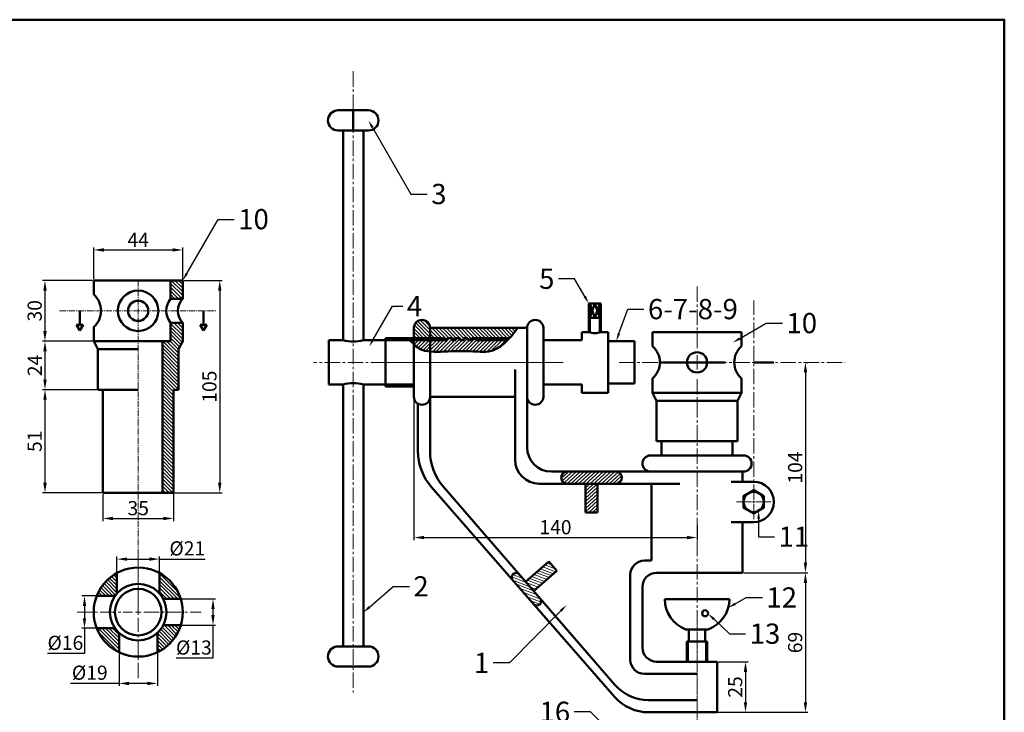
# Model space of a CAD drawing. Units: millimetres. Extents: x 434 to 1535, y -197 to 318.
# Tile 9 of 9: x 1049 to 1535, y -24 to 318. Entities that reach past the tile are written whole.
import ezdxf
from ezdxf import colors
from ezdxf.entities.mleader import LeaderData, LeaderLine
from ezdxf.math import Vec2, Vec3

# ---------------------------------------------------------------- set-up
doc = ezdxf.new("R2010")
doc.units = ezdxf.units.MM
doc.header["$LTSCALE"] = 0.4
doc.linetypes.add('CENTER2', pattern=[28.575, 19.05, -3.175, 3.175, -3.175])
doc.linetypes.add('DASHED', pattern=[19.05, 12.7, -6.35])
for name, color, linetype, lineweight in [('M-CNTR', 1, 'CENTER2', 18), ('M-DIMS', 2, 'Continuous', 25), ('M-HATC', 8, 'Continuous', 18), ('M-HIDN', 6, 'DASHED', 25), ('M-OUTL', 7, 'Continuous', 50), ('M-TEXT', 3, 'Continuous', 25)]:
    doc.layers.add(name, color=color, linetype=linetype, lineweight=lineweight)
doc.styles.get("Standard").update_dxf_attribs({"font": 'arial.ttf'})
doc.dimstyles.new('ISO-25', dxfattribs={"dimtxt": 7, "dimasz": 5, "dimexe": 1.25, "dimexo": 0.625, "dimtad": 1, "dimtoh": 1, "dimdec": 0, "dimtxsty": 'Standard', "dimcen": 2.5, "dimadec": 0, "dimazin": 0, "dimtfac": 1, "dimtdec": 0, "dimtmove": 0, "dimatfit": 3, "dimfxl": 1, "dimarcsym": 0})

# ---------------------------------------------------------------- blocks, each defined once
blk = doc.blocks.new('*U4')
at = {"layer": 'M-CNTR', "color": 0, "transparency": 16777216}
for p, q in [((0, 7), (0, 38.5)), ((-38.5, 0), (-7, 0)), ((7, 0), (73.2, 0)), ((0, -198.75), (0, -7))]:
    blk.add_line(p, q, dxfattribs=at)
at = {"layer": 'M-CNTR', "color": 0, "linetype": 'Continuous', "transparency": 16777216}
for p, q in [((-3.5, 0), (3.5, 0)), ((0, -3.5), (0, 3.5))]:
    blk.add_line(p, q, dxfattribs=at)
blk = doc.blocks.new('*U5')
at = {"layer": 'M-CNTR', "color": 0, "transparency": 16777216}
for p, q in [((0, 1), (0, 99.51)), ((-8.5, 0), (-1, 0)), ((1, 0), (8.5, 0)), ((0, -8.5), (0, -1))]:
    blk.add_line(p, q, dxfattribs=at)
at = {"layer": 'M-CNTR', "color": 0, "linetype": 'Continuous', "transparency": 16777216}
for p, q in [((-0.5, 0), (0.5, 0)), ((0, -0.5), (0, 0.5))]:
    blk.add_line(p, q, dxfattribs=at)
blk = doc.blocks.new('*U6')
at = {"layer": 'M-CNTR', "color": 0, "transparency": 16777216}
blk.add_line((-44.39, 0), (44.11, 0), dxfattribs=at)
blk = doc.blocks.new('*U46')
at = {"layer": 'M-CNTR', "color": 0, "transparency": 16777216}
blk.add_line((33.1, 0), (-82.84, 0), dxfattribs=at)
blk = doc.blocks.new('*U47')
at = {"layer": 'M-CNTR', "color": 0, "transparency": 16777216}
blk.add_line((0, 81.09), (0, -225.98), dxfattribs=at)
blk = doc.blocks.new('*U80')
at = {"layer": 'M-CNTR', "color": 0, "transparency": 16777216}
blk.add_line((0, -17.2), (0, 69.52), dxfattribs=at)
blk = doc.blocks.new('*D102')
at = {"layer": 'Defpoints', "color": 0, "ltscale": 0.4, "transparency": 16777216}
for p in [(1129.22, 204.63), (1085.22, 189.54), (1129.22, 189.54)]:
    blk.add_point(p, dxfattribs=at)
at = {"layer": 'M-DIMS', "color": 0, "lineweight": -2, "ltscale": 0.4, "transparency": 16777216}
for p, q in [((1085.22, 190.17), (1085.22, 205.88)), ((1090.22, 204.63), (1124.22, 204.63)), ((1129.22, 190.17), (1129.22, 205.88))]:
    blk.add_line(p, q, dxfattribs=at)
at = {"layer": 'M-DIMS', "color": 0, "ltscale": 0.4, "transparency": 16777216}
for points in [[(1090.22, 205.46), (1090.22, 203.79), (1085.22, 204.63)], [(1124.22, 205.46), (1124.22, 203.79), (1129.22, 204.63)]]:
    blk.add_solid(points, dxfattribs=at)
at = {"layer": 'M-DIMS', "color": 0, "ltscale": 0.4, "transparency": 16777216, "insert": (1107.22, 208.75), "char_height": 7, "attachment_point": 5}
blk.add_mtext('44', dxfattribs=at)
blk = doc.blocks.new('*D103')
at = {"layer": 'Defpoints', "color": 0, "ltscale": 0.4, "transparency": 16777216}
for p in [(1089.72, 84.54), (1124.72, 84.54), (1124.72, 71.88)]:
    blk.add_point(p, dxfattribs=at)
at = {"layer": 'M-DIMS', "color": 0, "lineweight": -2, "ltscale": 0.4, "transparency": 16777216}
for p, q in [((1089.72, 83.92), (1089.72, 70.63)), ((1124.72, 83.92), (1124.72, 70.63)), ((1094.72, 71.88), (1119.72, 71.88))]:
    blk.add_line(p, q, dxfattribs=at)
at = {"layer": 'M-DIMS', "color": 0, "ltscale": 0.4, "transparency": 16777216}
for points in [[(1094.72, 72.71), (1094.72, 71.05), (1089.72, 71.88)], [(1119.72, 72.71), (1119.72, 71.05), (1124.72, 71.88)]]:
    blk.add_solid(points, dxfattribs=at)
at = {"layer": 'M-DIMS', "color": 0, "ltscale": 0.4, "transparency": 16777216, "insert": (1107.22, 76.08), "char_height": 7, "attachment_point": 5}
blk.add_mtext('35', dxfattribs=at)
blk = doc.blocks.new('*D104')
at = {"layer": 'Defpoints', "color": 0, "ltscale": 0.4, "transparency": 16777216}
for p in [(1085.22, 189.54), (1061.12, 159.54), (1085.22, 159.54)]:
    blk.add_point(p, dxfattribs=at)
at = {"layer": 'M-DIMS', "color": 0, "lineweight": -2, "ltscale": 0.4, "transparency": 16777216}
for p, q in [((1084.6, 189.54), (1059.87, 189.54)), ((1061.12, 184.54), (1061.12, 164.54)), ((1084.6, 159.54), (1059.87, 159.54))]:
    blk.add_line(p, q, dxfattribs=at)
at = {"layer": 'M-DIMS', "color": 0, "ltscale": 0.4, "transparency": 16777216}
for points in [[(1060.29, 184.54), (1061.96, 184.54), (1061.12, 189.54)], [(1060.29, 164.54), (1061.96, 164.54), (1061.12, 159.54)]]:
    blk.add_solid(points, dxfattribs=at)
at = {"layer": 'M-DIMS', "color": 0, "ltscale": 0.4, "transparency": 16777216, "insert": (1056.92, 174.54), "char_height": 7, "attachment_point": 5, "rotation": 90}
blk.add_mtext('30', dxfattribs=at)
blk = doc.blocks.new('*D105')
at = {"layer": 'Defpoints', "color": 0, "ltscale": 0.4, "transparency": 16777216}
for p in [(1085.22, 159.54), (1061.12, 135.54), (1087.22, 135.54)]:
    blk.add_point(p, dxfattribs=at)
at = {"layer": 'M-DIMS', "color": 0, "lineweight": -2, "ltscale": 0.4, "transparency": 16777216}
for p, q in [((1084.6, 159.54), (1059.87, 159.54)), ((1061.12, 154.54), (1061.12, 140.54)), ((1086.6, 135.54), (1059.87, 135.54))]:
    blk.add_line(p, q, dxfattribs=at)
at = {"layer": 'M-DIMS', "color": 0, "ltscale": 0.4, "transparency": 16777216}
for points in [[(1060.29, 154.54), (1061.96, 154.54), (1061.12, 159.54)], [(1060.29, 140.54), (1061.96, 140.54), (1061.12, 135.54)]]:
    blk.add_solid(points, dxfattribs=at)
at = {"layer": 'M-DIMS', "color": 0, "ltscale": 0.4, "transparency": 16777216, "insert": (1056.98, 147.54), "char_height": 7, "attachment_point": 5, "rotation": 90}
blk.add_mtext('24', dxfattribs=at)
blk = doc.blocks.new('*D101')
at = {"layer": 'Defpoints', "color": 0, "ltscale": 0.4, "transparency": 16777216}
for p in [(1087.22, 135.54), (1061.12, 84.54), (1089.72, 84.54)]:
    blk.add_point(p, dxfattribs=at)
at = {"layer": 'M-DIMS', "color": 0, "lineweight": -2, "ltscale": 0.4, "transparency": 16777216}
for p, q in [((1086.6, 135.54), (1059.87, 135.54)), ((1061.12, 130.54), (1061.12, 89.54)), ((1089.1, 84.54), (1059.87, 84.54))]:
    blk.add_line(p, q, dxfattribs=at)
at = {"layer": 'M-DIMS', "color": 0, "ltscale": 0.4, "transparency": 16777216}
for points in [[(1060.29, 130.54), (1061.96, 130.54), (1061.12, 135.54)], [(1060.29, 89.54), (1061.96, 89.54), (1061.12, 84.54)]]:
    blk.add_solid(points, dxfattribs=at)
at = {"layer": 'M-DIMS', "color": 0, "ltscale": 0.4, "transparency": 16777216, "insert": (1056.92, 110.04), "char_height": 7, "attachment_point": 5, "rotation": 90}
blk.add_mtext('51', dxfattribs=at)
blk = doc.blocks.new('*D106')
at = {"layer": 'Defpoints', "color": 0, "ltscale": 0.4, "transparency": 16777216}
for p in [(1129.22, 189.54), (1119.22, 84.54), (1147.54, 84.54)]:
    blk.add_point(p, dxfattribs=at)
at = {"layer": 'M-DIMS', "color": 0, "lineweight": -2, "ltscale": 0.4, "transparency": 16777216}
for p, q in [((1129.85, 189.54), (1148.79, 189.54)), ((1147.54, 184.54), (1147.54, 89.54)), ((1119.85, 84.54), (1148.79, 84.54))]:
    blk.add_line(p, q, dxfattribs=at)
at = {"layer": 'M-DIMS', "color": 0, "ltscale": 0.4, "transparency": 16777216}
for points in [[(1146.71, 184.54), (1148.38, 184.54), (1147.54, 189.54)], [(1146.71, 89.54), (1148.38, 89.54), (1147.54, 84.54)]]:
    blk.add_solid(points, dxfattribs=at)
at = {"layer": 'M-DIMS', "color": 0, "ltscale": 0.4, "transparency": 16777216, "insert": (1143.34, 137.04), "char_height": 7, "attachment_point": 5, "rotation": 90}
blk.add_mtext('105', dxfattribs=at)
blk = doc.blocks.new('*U100')
at = {"layer": 'M-CNTR', "color": 0, "transparency": 16777216}
for p, q in [((0, 2.8), (0, 28.76)), ((-30.25, 0), (-2.8, 0)), ((2.8, 0), (31.18, 0)), ((0, -32.64), (0, -2.8))]:
    blk.add_line(p, q, dxfattribs=at)
at = {"layer": 'M-CNTR', "color": 0, "linetype": 'Continuous', "transparency": 16777216}
for p, q in [((-1.4, 0), (1.4, 0)), ((0, -1.4), (0, 1.4))]:
    blk.add_line(p, q, dxfattribs=at)
blk = doc.blocks.new('*D107')
at = {"layer": 'Defpoints', "color": 0, "ltscale": 0.4, "transparency": 16777216}
for p in [(1117.72, 51.8), (1096.72, 44.92), (1117.72, 44.92)]:
    blk.add_point(p, dxfattribs=at)
at = {"layer": 'M-DIMS', "color": 0, "lineweight": -2, "ltscale": 0.4, "transparency": 16777216}
for p, q in [((1096.72, 45.55), (1096.72, 53.05)), ((1101.72, 51.8), (1112.72, 51.8)), ((1117.72, 45.55), (1117.72, 53.05)), ((1117.72, 51.8), (1140.26, 51.8))]:
    blk.add_line(p, q, dxfattribs=at)
at = {"layer": 'M-DIMS', "color": 0, "ltscale": 0.4, "transparency": 16777216}
for points in [[(1101.72, 52.63), (1101.72, 50.96), (1096.72, 51.8)], [(1112.72, 52.63), (1112.72, 50.96), (1117.72, 51.8)]]:
    blk.add_solid(points, dxfattribs=at)
at = {"layer": 'M-DIMS', "color": 0, "ltscale": 0.4, "transparency": 16777216, "insert": (1131.49, 56.19), "char_height": 7, "attachment_point": 5}
blk.add_mtext('%%C21', dxfattribs=at)
blk = doc.blocks.new('*D108')
at = {"layer": 'Defpoints', "color": 0, "ltscale": 0.4, "transparency": 16777216}
for p in [(1128.24, 32.09), (1128.24, 19.09), (1144.19, 19.09)]:
    blk.add_point(p, dxfattribs=at)
at = {"layer": 'M-DIMS', "color": 0, "lineweight": -2, "ltscale": 0.4, "transparency": 16777216}
for p, q in [((1128.86, 32.09), (1145.44, 32.09)), ((1144.19, 27.09), (1144.19, 24.09)), ((1128.86, 19.09), (1145.44, 19.09)), ((1144.19, 19.09), (1144.19, 2.78)), ((1144.19, 2.78), (1125.92, 2.78))]:
    blk.add_line(p, q, dxfattribs=at)
at = {"layer": 'M-DIMS', "color": 0, "ltscale": 0.4, "transparency": 16777216}
for points in [[(1143.36, 27.09), (1145.02, 27.09), (1144.19, 32.09)], [(1143.36, 24.09), (1145.02, 24.09), (1144.19, 19.09)]]:
    blk.add_solid(points, dxfattribs=at)
at = {"layer": 'M-DIMS', "color": 0, "ltscale": 0.4, "transparency": 16777216, "insert": (1134.74, 7.18), "char_height": 7, "attachment_point": 5}
blk.add_mtext('%%C13', dxfattribs=at)
blk = doc.blocks.new('*D109')
at = {"layer": 'Defpoints', "color": 0, "ltscale": 0.4, "transparency": 16777216}
for p in [(1086.73, 33.59), (1080.65, 17.59), (1086.73, 17.59)]:
    blk.add_point(p, dxfattribs=at)
at = {"layer": 'M-DIMS', "color": 0, "lineweight": -2, "ltscale": 0.4, "transparency": 16777216}
for p, q in [((1086.1, 33.59), (1079.4, 33.59)), ((1080.65, 28.59), (1080.65, 22.59)), ((1086.1, 17.59), (1079.4, 17.59)), ((1080.65, 17.59), (1080.65, 5.11)), ((1080.65, 5.11), (1062.39, 5.11))]:
    blk.add_line(p, q, dxfattribs=at)
at = {"layer": 'M-DIMS', "color": 0, "ltscale": 0.4, "transparency": 16777216}
for points in [[(1079.82, 28.59), (1081.48, 28.59), (1080.65, 33.59)], [(1079.82, 22.59), (1081.48, 22.59), (1080.65, 17.59)]]:
    blk.add_solid(points, dxfattribs=at)
at = {"layer": 'M-DIMS', "color": 0, "ltscale": 0.4, "transparency": 16777216, "insert": (1071.21, 9.5), "char_height": 7, "attachment_point": 5}
blk.add_mtext('%%C16', dxfattribs=at)
blk = doc.blocks.new('*D110')
at = {"layer": 'Defpoints', "color": 0, "ltscale": 0.4, "transparency": 16777216}
for p in [(1097.72, 5.75), (1116.72, 5.75), (1116.72, -9.67)]:
    blk.add_point(p, dxfattribs=at)
at = {"layer": 'M-DIMS', "color": 0, "lineweight": -2, "ltscale": 0.4, "transparency": 16777216}
for p, q in [((1097.72, 5.12), (1097.72, -10.92)), ((1116.72, 5.12), (1116.72, -10.92)), ((1097.72, -9.67), (1073.81, -9.67)), ((1111.72, -9.67), (1102.72, -9.67))]:
    blk.add_line(p, q, dxfattribs=at)
at = {"layer": 'M-DIMS', "color": 0, "ltscale": 0.4, "transparency": 16777216}
for points in [[(1102.72, -8.83), (1102.72, -10.5), (1097.72, -9.67)], [(1111.72, -8.83), (1111.72, -10.5), (1116.72, -9.67)]]:
    blk.add_solid(points, dxfattribs=at)
at = {"layer": 'M-DIMS', "color": 0, "ltscale": 0.4, "transparency": 16777216, "insert": (1083.27, -5.27), "char_height": 7, "attachment_point": 5}
blk.add_mtext('%%C19', dxfattribs=at)
blk = doc.blocks.new('*D127')
at = {"layer": 'Defpoints', "color": 0, "ltscale": 0.4, "transparency": 16777216}
for p in [(1436.75, 149.06), (1406.04, 45.06), (1437.14, 45.06)]:
    blk.add_point(p, dxfattribs=at)
at = {"layer": 'M-DIMS', "color": 0, "lineweight": -2, "ltscale": 0.4, "transparency": 16777216}
for p, q in [((1437.38, 149.06), (1438.39, 149.06)), ((1437.14, 144.06), (1437.14, 50.06)), ((1406.66, 45.06), (1438.39, 45.06))]:
    blk.add_line(p, q, dxfattribs=at)
at = {"layer": 'M-DIMS', "color": 0, "ltscale": 0.4, "transparency": 16777216}
for points in [[(1436.31, 144.06), (1437.98, 144.06), (1437.14, 149.06)], [(1436.31, 50.06), (1437.98, 50.06), (1437.14, 45.06)]]:
    blk.add_solid(points, dxfattribs=at)
at = {"layer": 'M-DIMS', "color": 0, "ltscale": 0.4, "transparency": 16777216, "insert": (1432.95, 97.06), "char_height": 7, "attachment_point": 5, "rotation": 90}
blk.add_mtext('104', dxfattribs=at)
blk = doc.blocks.new('*D128')
at = {"layer": 'Defpoints', "color": 0, "ltscale": 0.4, "transparency": 16777216}
for p in [(1406.04, 45.06), (1383.54, -23.94), (1437.14, -23.94)]:
    blk.add_point(p, dxfattribs=at)
at = {"layer": 'M-DIMS', "color": 0, "lineweight": -2, "ltscale": 0.4, "transparency": 16777216}
for p, q in [((1406.66, 45.06), (1438.39, 45.06)), ((1437.14, 40.06), (1437.14, -18.94)), ((1384.16, -23.94), (1438.39, -23.94))]:
    blk.add_line(p, q, dxfattribs=at)
at = {"layer": 'M-DIMS', "color": 0, "ltscale": 0.4, "transparency": 16777216}
for points in [[(1436.31, 40.06), (1437.98, 40.06), (1437.14, 45.06)], [(1436.31, -18.94), (1437.98, -18.94), (1437.14, -23.94)]]:
    blk.add_solid(points, dxfattribs=at)
at = {"layer": 'M-DIMS', "color": 0, "ltscale": 0.4, "transparency": 16777216, "insert": (1432.95, 10.56), "char_height": 7, "attachment_point": 5, "rotation": 90}
blk.add_mtext('69', dxfattribs=at)
blk = doc.blocks.new('*D129')
at = {"layer": 'Defpoints', "color": 0, "ltscale": 0.4, "transparency": 16777216}
for p in [(1393.54, 1.06), (1393.54, -23.94), (1407.51, -23.94)]:
    blk.add_point(p, dxfattribs=at)
at = {"layer": 'M-DIMS', "color": 0, "lineweight": -2, "ltscale": 0.4, "transparency": 16777216}
for p, q in [((1394.16, 1.06), (1408.76, 1.06)), ((1407.51, -3.94), (1407.51, -18.94)), ((1394.16, -23.94), (1408.76, -23.94))]:
    blk.add_line(p, q, dxfattribs=at)
at = {"layer": 'M-DIMS', "color": 0, "ltscale": 0.4, "transparency": 16777216}
for points in [[(1406.67, -3.94), (1408.34, -3.94), (1407.51, 1.06)], [(1406.67, -18.94), (1408.34, -18.94), (1407.51, -23.94)]]:
    blk.add_solid(points, dxfattribs=at)
at = {"layer": 'M-DIMS', "color": 0, "ltscale": 0.4, "transparency": 16777216, "insert": (1403.31, -11.44), "char_height": 7, "attachment_point": 5, "rotation": 90}
blk.add_mtext('25', dxfattribs=at)
blk = doc.blocks.new('*D130')
at = {"layer": 'Defpoints', "color": 0, "ltscale": 0.4, "transparency": 16777216}
for p in [(1243.54, 137.06), (1383.54, 69.2), (1383.54, 62.45)]:
    blk.add_point(p, dxfattribs=at)
at = {"layer": 'M-DIMS', "color": 0, "lineweight": -2, "ltscale": 0.4, "transparency": 16777216}
for p, q in [((1243.54, 136.43), (1243.54, 61.2)), ((1383.54, 68.57), (1383.54, 61.2)), ((1248.54, 62.45), (1378.54, 62.45))]:
    blk.add_line(p, q, dxfattribs=at)
at = {"layer": 'M-DIMS', "color": 0, "ltscale": 0.4, "transparency": 16777216}
for points in [[(1248.54, 63.28), (1248.54, 61.62), (1243.54, 62.45)], [(1378.54, 63.28), (1378.54, 61.62), (1383.54, 62.45)]]:
    blk.add_solid(points, dxfattribs=at)
at = {"layer": 'M-DIMS', "color": 0, "ltscale": 0.4, "transparency": 16777216, "insert": (1313.54, 66.65), "char_height": 7, "attachment_point": 5}
blk.add_mtext('140', dxfattribs=at)
blk = doc.blocks.new('DIE')
at = {"ltscale": 0.4}
for p, q in [((0, 15), (32, 15)), ((21.57, 0), (10.43, 0))]:
    blk.add_line(p, q, dxfattribs=at)
for start, end in [(180, 249.6359), (290.3641, 0)]:
    blk.add_arc((16, 15), 16, start, end, dxfattribs=at)

msp = doc.modelspace()

# ---------------------------------------------------------------- hatches: boundary and pattern name
at = {"layer": 'M-HATC', "ltscale": 0.4}
h = msp.add_hatch(dxfattribs=at)
h.set_pattern_fill('ANSI31', color=256, scale=0.4, angle=90)
h.set_pattern_definition([(135, (-60.0056, 264.9336), (-0.8980256, -0.8980256), [])])
h.paths.add_polyline_path([(1119.22, 84.54), (1124.72, 84.54), (1124.72, 135.54), (1127.22, 135.54), (1127.22, 155.54), (1129.22, 159.54), (1129.22, 168.54), (1123.22, 168.54), (1123.22, 159.54), (1119.22, 159.54)])
h.paths.add_polyline_path([(1129.22, 189.54), (1123.22, 189.54), (1123.22, 180.54), (1129.22, 180.54)])
h = msp.add_hatch(dxfattribs=at)
h.set_pattern_fill('ANSI31', color=256, scale=0.4, angle=90)
h.set_pattern_definition([(135, (1944.4597, -517.0887), (-0.8980256, -0.8980256), [])])
edge = h.paths.add_edge_path()
edge.add_line((1251.54, 166.06), (1251.54, 161.06))
edge.add_line((1251.54, 161.06), (1258.22, 161.06))
edge.add_line((1258.22, 161.06), (1290.81, 161.06))
edge.add_spline(control_points=[(1290.81, 161.06), (1292.23, 162.63), (1293.6, 164.34), (1294.97, 166.06)], knot_values=[54.490486, 54.490486, 54.490486, 54.490486, 60.411943, 60.411943, 60.411943, 60.411943], degree=3, periodic=0)
edge.add_line((1294.97, 166.06), (1251.54, 166.06))
h.paths.add_polyline_path([(1251.54, 166.06, 1), (1243.54, 166.06), (1243.54, 161.06), (1251.54, 161.06)])
h = msp.add_hatch(dxfattribs=at)
h.set_pattern_fill('ANSI31', color=256, scale=0.4)
h.set_pattern_definition([(45, (1944.4597, -517.0887), (-0.8980256, 0.8980256), [])])
edge = h.paths.add_edge_path()
edge.add_spline(control_points=[(1251.54, 154.39), (1253.75, 154.19), (1261.99, 154.61), (1271.04, 154.74), (1282.58, 153.83), (1287.09, 157.16), (1289.88, 160.06)], knot_values=[13.163081, 13.163081, 13.163081, 13.163081, 19.718754, 36.150911, 41.776837, 53.205274, 53.205274, 53.205274, 53.205274], degree=3, periodic=0)
edge.add_line((1289.88, 160.06), (1278.04, 160.06))
edge.add_spline(control_points=[(1278.04, 160.06), (1277.22, 159.19), (1275.16, 156.98), (1270.08, 158.14), (1265.21, 158.03), (1260.18, 157.28), (1257.67, 159.16), (1256.48, 160.06)], knot_values=[0, 0, 0, 0, 3.382531, 8.59366, 13.864007, 18.596096, 22.91005, 22.91005, 22.91005, 22.91005], degree=3, periodic=0)
edge.add_line((1256.48, 160.06), (1251.54, 160.06))
edge.add_line((1251.54, 160.06), (1251.54, 154.39))
edge = h.paths.add_edge_path()
edge.add_line((1251.54, 160.06), (1243.54, 160.06))
edge.add_line((1243.54, 160.06), (1243.54, 157.99))
edge.add_spline(control_points=[(1243.54, 157.99), (1244.35, 157.17), (1246.66, 155.25), (1249.6, 154.57), (1251.54, 154.39)], knot_values=[3.982747, 3.982747, 3.982747, 3.982747, 7.427781, 13.163081, 13.163081, 13.163081, 13.163081], degree=3, periodic=0)
edge.add_line((1251.54, 154.39), (1251.54, 160.06))
edge = h.paths.add_edge_path()
edge.add_spline(control_points=[(1256.48, 160.06), (1257.67, 159.16), (1260.18, 157.28), (1265.21, 158.03), (1270.08, 158.14), (1275.16, 156.98), (1277.22, 159.19), (1278.04, 160.06)], knot_values=[0, 0, 0, 0, 4.313954, 9.046043, 14.31639, 19.527519, 22.91005, 22.91005, 22.91005, 22.91005], degree=3, periodic=0)
edge.add_line((1278.04, 160.06), (1274.22, 160.06))
edge.add_line((1274.22, 160.06), (1274.22, 161.06))
edge.add_line((1274.22, 161.06), (1272.22, 161.06))
edge.add_line((1272.22, 161.06), (1272.22, 160.06))
edge.add_line((1272.22, 160.06), (1270.22, 160.06))
edge.add_line((1270.22, 160.06), (1270.22, 161.06))
edge.add_line((1270.22, 161.06), (1268.22, 161.06))
edge.add_line((1268.22, 161.06), (1268.22, 160.06))
edge.add_line((1268.22, 160.06), (1266.22, 160.06))
edge.add_line((1266.22, 160.06), (1266.22, 161.06))
edge.add_line((1266.22, 161.06), (1264.22, 161.06))
edge.add_line((1264.22, 161.06), (1264.22, 160.06))
edge.add_line((1264.22, 160.06), (1262.22, 160.06))
edge.add_line((1262.22, 160.06), (1262.22, 161.06))
edge.add_line((1262.22, 161.06), (1260.22, 161.06))
edge.add_line((1260.22, 161.06), (1260.22, 160.06))
edge.add_line((1260.22, 160.06), (1258.22, 160.06))
edge.add_line((1258.22, 160.06), (1256.48, 160.06))
h = msp.add_hatch(dxfattribs=at)
h.set_pattern_fill('ANSI31', color=256, scale=0.4, angle=177)
h.set_pattern_definition([(222, (735.9605, -22.5014), (0.8497959, -0.943794), [])])
h.paths.add_polyline_path([(1343.38, 95.06), (1319.38, 95.06, 1), (1319.38, 89.06), (1343.38, 89.06, 1)])
h.paths.add_polyline_path([(1334.38, 89.06), (1328.38, 89.06), (1328.38, 74.88), (1334.38, 74.88)])
h = msp.add_hatch(dxfattribs=at)
h.set_pattern_fill('ANSI31', color=256, scale=0.4, angle=114)
h.set_pattern_definition([(159, (735.9605, -22.5014), (-0.4551273, -1.1856471), [])])
h.paths.add_polyline_path([(1314.18, 46.03), (1310.23, 50.54), (1298.8, 40.56), (1302.74, 36.02)])
h.paths.add_polyline_path([(1302.78, 29.56, 0.998098), (1305.95, 32.32), (1295.62, 44.23, 1.001905), (1292.4, 41.43)])
h = msp.add_hatch(dxfattribs=at)
h.set_pattern_fill('ANSI31', color=256, scale=0.4, angle=90)
h.set_pattern_definition([(135, (-250.1834, 254.1624), (-0.8980256, -0.8980256), [])])
h.paths.add_polyline_path([(1128.24, 32.09, 0.195774), (1117.72, 44.92), (1117.72, 34.85, -0.060049), (1119.62, 32.09)])
h.paths.add_polyline_path([(1086.73, 33.59), (1095.73, 33.59, -0.02863), (1096.72, 34.85), (1096.72, 44.92, 0.177087)])
h.paths.add_polyline_path([(1097.72, 5.75), (1097.72, 15.31, -0.054237), (1095.73, 17.59), (1086.73, 17.59, 0.190278)])
h.paths.add_polyline_path([(1116.72, 5.75, 0.209058), (1128.24, 19.09), (1119.62, 19.09, -0.085747), (1116.72, 15.31)])

# ---------------------------------------------------------------- linework, layer by layer
at = {"layer": 'M-CNTR', "ltscale": 0.4}
for p, q in [((1107.22, 189.54), (1107.22, 25.59)), ((1068.34, 174.54), (1145.99, 174.54))]:
    msp.add_line(p, q, dxfattribs=at)
at = {"layer": 'M-HIDN', "ltscale": 0.4}
msp.add_line((1243.54, 161.06), (1290.81, 161.06), dxfattribs=at)
at = {"layer": 'M-OUTL', "ltscale": 0.4}
for p, q in [((1213.54, 273.67), (1213.54, 263.67)), ((1213.54, 263.67), (1208.54, 263.67)), ((1208.54, 263.67), (1208.54, 160.06)), ((1213.54, 263.67), (1218.54, 263.67)), ((1218.54, 263.67), (1218.54, 160.06)), ((1085.22, 189.54), (1129.22, 189.54)), ((1085.22, 182.54), (1085.22, 189.54)), ((1123.22, 180.54), (1123.22, 189.54)), ((1129.22, 189.54), (1129.22, 180.54)), ((1129.22, 180.54), (1123.22, 180.54)), ((1330.04, 178.14), (1330.04, 164.06)), ((1336.04, 178.14), (1330.04, 178.14)), ((1330.54, 178.14), (1330.54, 163.88)), ((1333.04, 171.14), (1330.54, 178.14)), ((1333.04, 178.14), (1330.54, 171.14)), ((1335.54, 178.14), (1333.04, 171.14)), ((1333.04, 178.14), (1335.54, 171.14)), ((1335.54, 163.88), (1335.54, 178.14)), ((1336.04, 164.06), (1336.04, 178.14)), ((1078.4, 174.54), (1078.4, 167.67)), ((1139.57, 174.54), (1139.57, 167.67)), ((1336.04, 171.14), (1330.04, 171.14)), ((1078.4, 164.8), (1076.74, 167.67)), ((1076.74, 167.67), (1080.05, 167.67)), ((1078.4, 164.8), (1080.05, 167.67)), ((1085.22, 159.54), (1085.22, 166.54)), ((1123.22, 159.54), (1123.22, 168.54)), ((1129.22, 168.54), (1123.22, 168.54)), ((1129.22, 168.54), (1129.22, 159.54)), ((1139.57, 164.8), (1137.91, 167.67)), ((1137.91, 167.67), (1141.23, 167.67)), ((1139.57, 164.8), (1141.23, 167.67)), ((1243.54, 132.06), (1243.54, 166.06)), ((1251.54, 166.06), (1251.54, 132.06)), ((1251.54, 166.06), (1299.54, 166.06)), ((1299.54, 132.06), (1299.54, 166.06)), ((1307.54, 166.06), (1307.54, 132.06)), ((1229.54, 161.06), (1229.54, 137.06)), ((1258.22, 161.06), (1229.54, 161.06)), ((1258.22, 161.06), (1258.22, 160.06)), ((1262.22, 161.06), (1260.22, 161.06)), ((1260.22, 160.06), (1260.22, 161.06)), ((1262.22, 161.06), (1262.22, 160.06)), ((1266.22, 161.06), (1264.22, 161.06)), ((1264.22, 160.06), (1264.22, 161.06)), ((1264.22, 161.06), (1266.22, 161.06)), ((1266.22, 161.06), (1266.22, 160.06)), ((1270.22, 161.06), (1268.22, 161.06)), ((1268.22, 160.06), (1268.22, 161.06)), ((1268.22, 161.06), (1270.22, 161.06)), ((1270.22, 161.06), (1270.22, 160.06)), ((1290.81, 161.06), (1272.22, 161.06)), ((1272.22, 160.06), (1272.22, 161.06)), ((1272.22, 161.06), (1274.22, 161.06)), ((1274.22, 161.06), (1274.22, 160.06)), ((1299.54, 137.06), (1299.54, 161.06)), ((1326.54, 164.06), (1326.54, 160.06)), ((1330.04, 164.06), (1326.54, 164.06)), ((1339.54, 164.06), (1336.04, 164.06)), ((1339.54, 149.06), (1339.54, 164.06)), ((1361.54, 164.06), (1405.54, 164.06)), ((1361.54, 157.06), (1361.54, 164.06)), ((1405.54, 164.06), (1405.54, 157.06)), ((1123.22, 159.54), (1085.22, 159.54)), ((1085.22, 159.54), (1087.22, 155.54)), ((1119.22, 159.54), (1119.22, 84.54)), ((1129.22, 159.54), (1127.22, 155.54)), ((1208.54, 160.06), (1201.54, 160.06)), ((1201.54, 160.06), (1201.54, 138.06)), ((1229.54, 160.06), (1218.54, 160.06)), ((1260.22, 160.06), (1229.54, 160.06)), ((1258.22, 160.06), (1260.22, 160.06)), ((1264.22, 160.06), (1262.22, 160.06)), ((1262.22, 160.06), (1264.22, 160.06)), ((1268.22, 160.06), (1266.22, 160.06)), ((1266.22, 160.06), (1268.22, 160.06)), ((1272.22, 160.06), (1270.22, 160.06)), ((1270.22, 160.06), (1272.22, 160.06)), ((1289.88, 160.06), (1274.22, 160.06)), ((1326.54, 160.06), (1307.54, 160.06)), ((1339.54, 159.56), (1339.54, 138.56)), ((1339.54, 159.56), (1352.54, 159.56)), ((1352.54, 138.56), (1352.54, 159.56)), ((1107.22, 155.54), (1087.22, 155.54)), ((1087.22, 135.54), (1087.22, 155.54)), ((1127.22, 155.54), (1127.22, 135.54)), ((1339.54, 134.06), (1339.54, 149.06)), ((1365.15, 149.06), (1397.42, 149.06)), ((1293.54, 145.49), (1293.54, 101.06)), ((1201.54, 138.06), (1208.54, 138.06)), ((1208.54, 138.06), (1208.54, 8.67)), ((1218.54, 138.06), (1229.54, 138.06)), ((1218.54, 138.06), (1218.54, 8.67)), ((1229.54, 138.06), (1243.54, 138.06)), ((1229.54, 137.06), (1243.54, 137.06)), ((1307.54, 138.06), (1326.54, 138.06)), ((1326.54, 138.06), (1326.54, 134.06)), ((1339.54, 138.56), (1352.54, 138.56)), ((1361.54, 134.06), (1361.54, 141.06)), ((1405.54, 134.06), (1405.54, 141.06)), ((1107.22, 135.54), (1087.22, 135.54)), ((1089.72, 135.54), (1089.72, 84.54)), ((1127.22, 135.54), (1124.72, 135.54)), ((1124.72, 135.54), (1124.72, 84.54)), ((1251.54, 132.06), (1293.54, 132.06)), ((1251.54, 105.14), (1251.54, 132.06)), ((1299.54, 132.06), (1299.54, 107.06)), ((1326.54, 134.06), (1339.54, 134.06)), ((1339.54, 134.06), (1333.54, 134.06)), ((1405.54, 134.06), (1361.54, 134.06)), ((1361.54, 134.06), (1363.54, 130.06)), ((1405.54, 134.06), (1403.54, 130.06)), ((1245.54, 105.19), (1245.54, 128.6)), ((1383.54, 130.06), (1363.54, 130.06)), ((1363.54, 110.06), (1363.54, 130.06)), ((1383.54, 130.06), (1403.54, 130.06)), ((1403.54, 110.06), (1403.54, 130.06)), ((1383.54, 110.06), (1363.54, 110.06)), ((1366.04, 110.06), (1366.04, 103.06)), ((1383.54, 110.06), (1403.54, 110.06)), ((1401.04, 110.06), (1401.04, 103.06)), ((1383.54, 95.06), (1311.54, 95.06)), ((1375.1, 89.06), (1305.54, 89.06)), ((1328.38, 89.06), (1328.38, 74.88)), ((1334.38, 89.06), (1334.38, 74.88)), ((1089.72, 84.54), (1124.72, 84.54)), ((1252.21, 87.43), (1342.96, -16.42)), ((1342.96, -10.35), (1258.14, 87.45)), ((1328.38, 74.88), (1334.38, 74.88)), ((1298.8, 40.56), (1310.23, 50.54)), ((1310.23, 50.54), (1314.18, 46.03)), ((1357.54, 51.06), (1361.04, 51.06)), ((1096.72, 44.92), (1096.72, 34.85)), ((1117.72, 44.92), (1117.72, 34.85)), ((1302.74, 36.02), (1314.18, 46.03)), ((1350.54, 44.06), (1350.54, 2.06)), ((1356.54, 38.06), (1356.54, 8.06)), ((1095.73, 33.59), (1086.73, 33.59)), ((1119.62, 32.09), (1128.24, 32.09)), ((1095.73, 17.59), (1086.73, 17.59)), ((1097.72, 15.31), (1097.72, 5.75)), ((1116.72, 15.31), (1116.72, 5.75)), ((1119.62, 19.09), (1128.24, 19.09)), ((1387.54, 17.03), (1379.54, 17.03)), ((1379.54, 17.03), (1379.54, 11.03)), ((1387.54, 11.03), (1387.54, 17.03)), ((1388.54, 11.03), (1378.54, 11.03)), ((1378.54, 1.06), (1378.54, 11.03)), ((1379.04, 1.06), (1379.04, 11.03)), ((1388.04, 1.06), (1388.04, 11.03)), ((1388.54, 1.06), (1388.54, 11.03)), ((1393.54, 1.06), (1393.54, -23.94)), ((1357.54, -4.94), (1383.54, -4.94)), ((1359.58, -17.94), (1383.54, -17.94))]:
    msp.add_line(p, q, dxfattribs=at)
at = {"layer": 'M-OUTL'}
for p, q in [((1411.54, 149.06), (1421.54, 149.06)), ((1406.04, 90.06), (1406.04, 95.06)), ((1361.04, 51.06), (1361.04, 89.06)), ((1411.54, 90.06), (1400.49, 90.06)), ((1411.54, 70.06), (1400.42, 70.06)), ((1406.04, 45.06), (1406.04, 70.06)), ((1406.04, 45.06), (1363.54, 45.06)), ((1383.54, 45.06), (1363.54, 45.06)), ((1363.54, 1.06), (1393.54, 1.06)), ((1373.54, 1.06), (1393.54, 1.06)), ((1359.53, -23.94), (1393.54, -23.94))]:
    msp.add_line(p, q, dxfattribs=at)
at = {"layer": 'M-OUTL', "ltscale": 0.4}
for points in [[(434.2, 318.45), (1535.47, 318.45), (1535.47, -197.48), (434.2, -197.48)], [(1416.54, 82.95), (1411.54, 85.83), (1406.54, 82.95), (1406.54, 77.17), (1411.54, 74.29), (1416.54, 77.17)]]:
    msp.add_lwpolyline(points, close=True, dxfattribs=at)
for points in [[(1206.04, 273.67, 1), (1206.04, 263.67), (1221.04, 263.67, 1), (1221.04, 273.67)], [(1206.04, 8.67, 1), (1206.04, -1.33), (1221.04, -1.33, 1), (1221.04, 8.67)]]:
    msp.add_lwpolyline(points, format="xyb", close=True, dxfattribs=at)
at = {"layer": 'M-OUTL'}
msp.add_lwpolyline([(1360.54, 103.06, 1), (1360.54, 95.06), (1406.54, 95.06, 1), (1406.54, 103.06), (1383.54, 103.06)], format="xyb", close=True, dxfattribs=at)
at = {"layer": 'M-OUTL', "ltscale": 0.4}
for centre, radius in [((1107.17, 174.54), 10), ((1107.17, 174.54), 5), ((1383.54, 149.06), 5), ((1107.22, 25.59), 22), ((1107.22, 25.59), 14), ((1107.22, 25.59), 11.5), ((1387.54, 25.03), 1.5)]:
    msp.add_circle(centre, radius, dxfattribs=at)
at = {"layer": 'M-OUTL'}
msp.add_circle((1411.54, 80.06), 5, dxfattribs=at)
at = {"layer": 'M-OUTL', "ltscale": 0.4}
for centre, radius, start, end in [((1078.17, 174.54), 10.66, 311.3764, 48.6236), ((1130.69, 174.54), 9.58, 141.2197, 218.7803), ((1135.58, 174.54), 8.74, 136.6674, 223.3326), ((1247.54, 166.06), 4, 0, 180), ((1303.54, 166.06), 4, 0, 180), ((1333.04, 171.46), 7.99, 247.9403, 292.0597), ((1213.54, 176.31), 17, 252.8954, 287.1046), ((1354.49, 149.06), 10.66, 311.3764, 48.6236), ((1412.58, 149.06), 10.66, 131.3764, 228.6236), ((1213.54, 121.81), 17, 72.8954, 107.1046), ((1247.54, 132.06), 4, 180, 0), ((1303.54, 132.06), 4, 180, 0), ((1272.54, 105.19), 27, 180, 221.1518), ((1278.54, 105.14), 27, 180, 220.9337), ((1311.54, 107.06), 12, 180, 270), ((1305.54, 101.06), 12, 180, 270), ((1319.38, 92.06), 3, 90, 270), ((1343.38, 92.06), 3, 270, 90), ((1357.54, 44.06), 7, 90, 180), ((1294.01, 42.83), 2.13, 40.9337, 221.1518), ((1363.54, 38.06), 7, 90, 180), ((1304.36, 30.94), 2.1, 221.1518, 40.9337), ((1357.54, 2.06), 7, 180, 270), ((1359.58, 4.06), 22, 220.9337, 270)]:
    msp.add_arc(centre, radius, start, end, dxfattribs=at)
at = {"layer": 'M-OUTL'}
for centre, radius, start, end in [((1411.54, 80.06), 10, 270, 90), ((1363.54, 8.06), 7, 180, 270), ((1359.53, -1.94), 22, 221.1518, 270)]:
    msp.add_arc(centre, radius, start, end, dxfattribs=at)
at = {"layer": 'M-OUTL', "ltscale": 0.4}
msp.add_open_spline([(1240.83, 161.06), (1242.47, 159.07), (1246.84, 153.79), (1260.18, 154.58), (1271.04, 154.74), (1285.06, 153.63), (1290.66, 160.66), (1294.97, 166.06)], degree=3, knots=[0, 0, 0, 0, 7.427781, 19.718754, 36.150911, 41.776837, 60.411943, 60.411943, 60.411943, 60.411943], dxfattribs=at)

# ---------------------------------------------------------------- block references
at = {"layer": 'M-CNTR'}
for name, p in [('*U47', (1213.54, 211.86)), ('*U4', (1383.54, 149.06)), ('*U5', (1411.54, 80.06)), ('*U46', (1276.79, 149.06)), ('*U6', (1274.04, 149.06)), ('*U100', (1107.22, 25.59)), ('*U80', (1383.54, -42.97))]:
    msp.add_blockref(name, p, dxfattribs=at)
at = {"layer": 'M-OUTL'}
msp.add_blockref('DIE', (1367.54, 17.03), dxfattribs=at)

# ---------------------------------------------------------------- dimensions: what is measured, and where the dimension line sits
at = {"layer": 'M-DIMS', "ltscale": 0.4}
for base, p1, p2, picture, middle in [((1129.22, 204.63), (1085.22, 189.54), (1129.22, 189.54), '*D102', (1107.22, 208.75)), ((1383.54, 62.45), (1243.54, 137.06), (1383.54, 69.2), '*D130', (1313.54, 66.65)), ((1124.72, 71.88), (1089.72, 84.54), (1124.72, 84.54), '*D103', (1107.22, 76.08))]:
    dim = msp.add_linear_dim(base=base, p1=p1, p2=p2, dimstyle='ISO-25', override={"dimclrd": 0, "dimclre": 0, "dimclrt": 0}, dxfattribs=at)
    dim.commit()
    dim.dimension.update_dxf_attribs({"geometry": picture, "text_midpoint": middle})
for base, p1, p2, picture, middle in [((1061.12, 159.54), (1085.22, 189.54), (1085.22, 159.54), '*D104', (1056.92, 174.54)), ((1147.54, 84.54), (1129.22, 189.54), (1119.22, 84.54), '*D106', (1143.34, 137.04)), ((1061.12, 135.54), (1085.22, 159.54), (1087.22, 135.54), '*D105', (1056.98, 147.54)), ((1437.14, 45.06), (1436.75, 149.06), (1406.04, 45.06), '*D127', (1432.95, 97.06)), ((1061.12, 84.54), (1087.22, 135.54), (1089.72, 84.54), '*D101', (1056.92, 110.04)), ((1437.14, -23.94), (1406.04, 45.06), (1383.54, -23.94), '*D128', (1432.95, 10.56)), ((1407.51, -23.94), (1393.54, 1.06), (1393.54, -23.94), '*D129', (1403.31, -11.44))]:
    dim = msp.add_linear_dim(base=base, p1=p1, p2=p2, angle=90, dimstyle='ISO-25', override={"dimclrd": 0, "dimclre": 0, "dimclrt": 0}, dxfattribs=at)
    dim.commit()
    dim.dimension.update_dxf_attribs({"geometry": picture, "text_midpoint": middle})
for base, p1, p2, picture, middle in [((1117.72, 51.8), (1096.72, 44.92), (1117.72, 44.92), '*D107', (1131.49, 51.8)), ((1116.72, -9.67), (1097.72, 5.75), (1116.72, 5.75), '*D110', (1083.27, -9.67))]:
    dim = msp.add_linear_dim(base=base, p1=p1, p2=p2, text='%%C<>', dimstyle='ISO-25', override={"dimclrd": 0, "dimclre": 0, "dimclrt": 0}, dxfattribs=at)
    dim.commit()
    dim.dimension.update_dxf_attribs({"geometry": picture, "text_midpoint": middle, "dimtype": 160})
for base, p1, p2, picture, middle in [((1080.65, 17.59), (1086.73, 33.59), (1086.73, 17.59), '*D109', (1071.21, 5.11)), ((1144.19, 19.09), (1128.24, 32.09), (1128.24, 19.09), '*D108', (1134.74, 2.78))]:
    dim = msp.add_linear_dim(base=base, p1=p1, p2=p2, angle=90, text='%%C<>', dimstyle='ISO-25', override={"dimclrd": 0, "dimclre": 0, "dimclrt": 0}, dxfattribs=at)
    dim.commit()
    dim.dimension.update_dxf_attribs({"geometry": picture, "text_midpoint": middle, "dimtype": 160})

# ---------------------------------------------------------------- leaders
at = {"layer": 'M-TEXT', "ltscale": 0.4}
ml = msp.add_multileader_mtext('Standard', dxfattribs=at)
ml.set_content('3', color=256)
ml.set_leader_properties()
ml.build(insert=Vec2(0, 0))
ctx = ml.context
ctx.base_point, ctx.char_height, ctx.plane_origin = Vec3(1250.1, 232.18), 10, Vec3(1221.04, 268.67)
notes = []
notes.append((ctx, [(0, (1, 1, 0), (1242.1, 232.18), (1, 0), 8, [(0, [(1221.04, 268.67)], 0, [])])]))
ctx.mtext.insert, ctx.mtext.flow_direction = Vec3(1252.1, 237.27), 5
ml = msp.add_multileader_mtext('Standard', dxfattribs=at)
ml.set_content('10', color=256)
ml.set_leader_properties()
ml.build(insert=Vec2(0, 0))
ctx = ml.context
ctx.base_point, ctx.char_height, ctx.plane_origin = Vec3(1154.67, 219.76), 10, Vec3(1129.22, 189.54)
notes.append((ctx, [(0, (1, 1, 0), (1146.67, 219.76), (1, 0), 8, [(0, [(1129.22, 189.54)], 0, [])])]))
ctx.mtext.insert, ctx.mtext.flow_direction = Vec3(1156.67, 224.85), 5
ml = msp.add_multileader_mtext('Standard', dxfattribs=at)
ml.set_content('5', color=256)
ml.set_leader_properties()
ml.build(insert=Vec2(0, 0))
ctx = ml.context
ctx.base_point, ctx.char_height, ctx.plane_origin = Vec3(1304.39, 190.3), 10, Vec3(1330.04, 178.14)
ctx.text_align_type = 2
notes.append((ctx, [(0, (1, 1, 0), (1323.02, 190.3), (-1, 0), 8, [(0, [(1330.04, 178.14)], 0, [])])]))
ctx.mtext.insert, ctx.mtext.alignment, ctx.mtext.flow_direction = Vec3(1313.02, 195.38), 3, 5
ml = msp.add_multileader_mtext('Standard', dxfattribs=at)
ml.set_content('4', color=256)
ml.set_leader_properties()
ml.build(insert=Vec2(0, 0))
ctx = ml.context
ctx.base_point, ctx.char_height, ctx.plane_origin = Vec3(1238.02, 176.82), 10, Vec3(1221.42, 156.9)
notes.append((ctx, [(0, (1, 1, 0), (1232.92, 176.82), (1, 0), 5.1, [(0, [(1221.42, 156.9)], 0, [])])]))
ctx.mtext.insert, ctx.mtext.flow_direction = Vec3(1240.02, 181.82), 5
ml = msp.add_multileader_mtext('Standard', dxfattribs=at)
ml.set_content('6-7-8-9', color=256)
ml.set_leader_properties()
ml.build(insert=Vec2(0, 0))
ctx = ml.context
ctx.base_point, ctx.char_height, ctx.plane_origin = Vec3(1357.25, 175.31), 10, Vec3(1343.57, 159.56)
notes.append((ctx, [(0, (1, 1, 0), (1349.25, 175.31), (1, 0), 8, [(0, [(1343.57, 159.56)], 0, [])])]))
ctx.mtext.insert, ctx.mtext.flow_direction = Vec3(1359.25, 180.39), 5
ml = msp.add_multileader_mtext('Standard', dxfattribs=at)
ml.set_content('10', color=256)
ml.set_leader_properties()
ml.build(insert=Vec2(0, 0))
ctx = ml.context
ctx.base_point, ctx.char_height, ctx.plane_origin = Vec3(1425.76, 168.38), 10, Vec3(1401.2, 158.82)
notes.append((ctx, [(0, (1, 1, 0), (1417.76, 168.38), (1, 0), 8, [(0, [(1401.2, 158.82)], 0, [])])]))
ctx.mtext.insert, ctx.mtext.flow_direction = Vec3(1427.76, 173.47), 5
ml = msp.add_multileader_mtext('Standard', dxfattribs=at)
ml.set_content('11', color=256)
ml.set_leader_properties()
ml.build(insert=Vec2(0, 0))
ctx = ml.context
ctx.base_point, ctx.char_height, ctx.plane_origin = Vec3(1421.85, 62.87), 10, Vec3(1414.04, 75.73)
notes.append((ctx, [(0, (1, 1, 0), (1413.85, 62.87), (1, 0), 8, [(0, [(1414.04, 75.73)], 0, [])])]))
ctx.mtext.insert, ctx.mtext.flow_direction = Vec3(1423.85, 67.87), 5
ml = msp.add_multileader_mtext('Standard', dxfattribs=at)
ml.set_content('2', color=256)
ml.set_leader_properties()
ml.build(insert=Vec2(0, 0))
ctx = ml.context
ctx.base_point, ctx.char_height, ctx.plane_origin = Vec3(1241.28, 38.31), 10, Vec3(1218.54, 25.43)
notes.append((ctx, [(0, (1, 1, 0), (1233.28, 38.31), (1, 0), 8, [(0, [(1218.54, 25.43)], 0, [])])]))
ctx.mtext.insert, ctx.mtext.flow_direction = Vec3(1243.28, 43.31), 5
ml = msp.add_multileader_mtext('Standard', dxfattribs=at)
ml.set_content('12', color=256)
ml.set_leader_properties()
ml.build(insert=Vec2(0, 0))
ctx = ml.context
ctx.base_point, ctx.char_height, ctx.plane_origin = Vec3(1415.83, 32.83), 10, Vec3(1398.94, 27.7)
notes.append((ctx, [(0, (1, 1, 0), (1407.83, 32.83), (1, 0), 8, [(0, [(1398.94, 27.7)], 0, [])])]))
ctx.mtext.insert, ctx.mtext.flow_direction = Vec3(1417.83, 37.83), 5
ml = msp.add_multileader_mtext('Standard', dxfattribs=at)
ml.set_content('1', color=256)
ml.set_leader_properties()
ml.build(insert=Vec2(0, 0))
ctx = ml.context
ctx.base_point, ctx.char_height, ctx.plane_origin = Vec3(1275.05, 0.51), 10, Vec3(1319.02, 29.05)
ctx.text_align_type = 2
notes.append((ctx, [(0, (1, 1, 0), (1290.74, 0.51), (-1, 0), 8, [(0, [(1319.02, 29.05)], 0, [])])]))
ctx.mtext.insert, ctx.mtext.alignment, ctx.mtext.flow_direction = Vec3(1280.74, 5.51), 3, 5
ml = msp.add_multileader_mtext('Standard', dxfattribs=at)
ml.set_content('13', color=256)
ml.set_leader_properties()
ml.build(insert=Vec2(0, 0))
ctx = ml.context
ctx.base_point, ctx.char_height, ctx.plane_origin = Vec3(1407.58, 14.85), 10, Vec3(1389.02, 24.79)
notes.append((ctx, [(0, (1, 1, 0), (1399.58, 14.85), (1, 0), 8, [(0, [(1389.02, 24.79)], 0, [])])]))
ctx.mtext.insert, ctx.mtext.flow_direction = Vec3(1409.58, 19.94), 5
ml = msp.add_multileader_mtext('Standard', dxfattribs=at)
ml.set_content('16', color=256)
ml.set_leader_properties()
ml.build(insert=Vec2(0, 0))
ctx = ml.context
ctx.base_point, ctx.char_height, ctx.plane_origin = Vec3(1305.43, -23.78), 10, Vec3(1343.94, -37)
ctx.text_align_type = 2
notes.append((ctx, [(0, (1, 1, 0), (1330.8, -23.78), (-1, 0), 8, [(0, [(1343.94, -37)], 0, [])])]))
ctx.mtext.insert, ctx.mtext.alignment, ctx.mtext.flow_direction = Vec3(1320.8, -18.7), 3, 5
for ctx, leaders in notes:
    for number, flags, end, landing, length, lines in leaders:
        leader = LeaderData()
        leader.index, (leader.has_last_leader_line, leader.has_dogleg_vector, leader.attachment_direction) = number, flags
        leader.last_leader_point, leader.dogleg_vector, leader.dogleg_length = Vec3(end), Vec3(landing), length
        for number, points, colour, breaks in lines:
            line = LeaderLine()
            line.index, line.vertices, line.color, line.breaks = number, Vec3.list(points), colors.encode_raw_color(colour), breaks
            leader.lines.append(line)
        ctx.leaders.append(leader)

doc.saveas('drawing.dxf')
